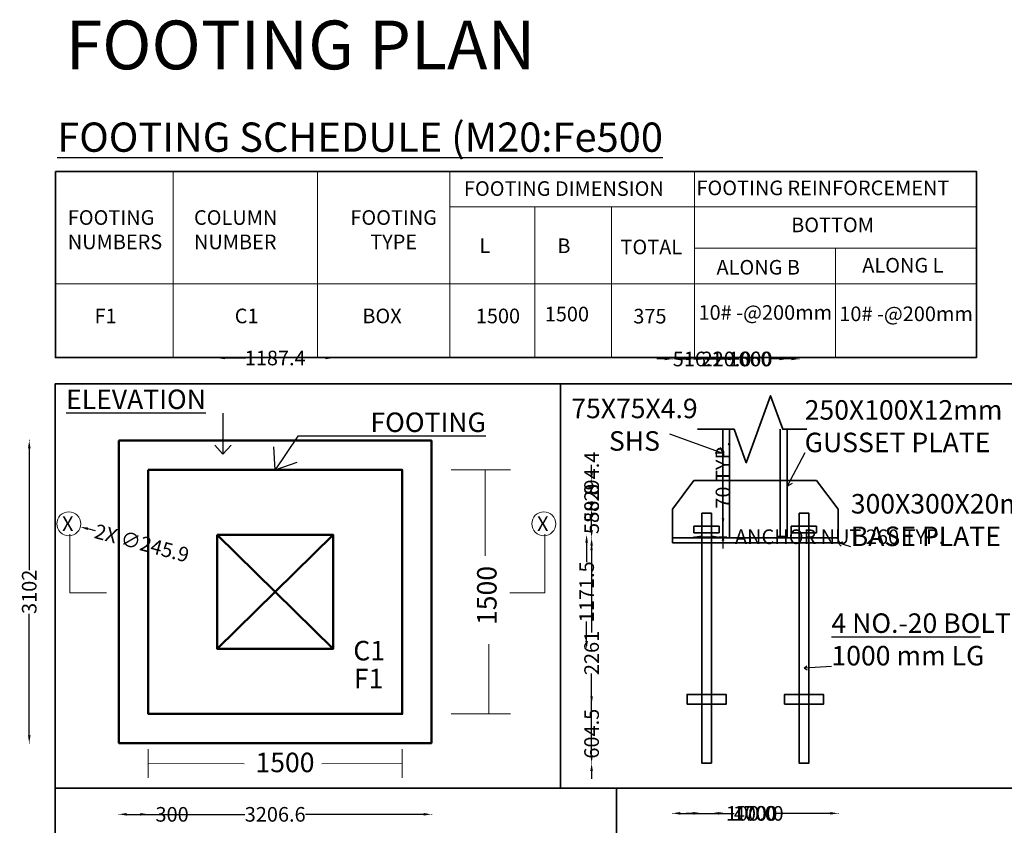
# Model space of a CAD drawing. Units: millimetres. Extents: x -19888 to 14444, y 67066 to 90098.
# Tile 2 of 7: x -19617 to -9513, y 73856 to 82117. Entities that reach past the tile are written whole.
import ezdxf

# ---------------------------------------------------------------- set-up
doc = ezdxf.new("R2010")
doc.units = ezdxf.units.MM
doc.header["$LTSCALE"] = 50
doc.header["$MEASUREMENT"] = 0
for name, color, linetype, lineweight in [('S-ANNO-DIMS', 2, 'Continuous', 18), ('S-ANNO-SYMB', 3, 'Continuous', 18), ('S-ANNO-TABL', 7, 'Continuous', 18), ('S-ANNO-TEXT', 7, 'Continuous', 25), ('S-ANNO-TTLB', 7, 'Continuous', 35), ('S-COLS', 4, 'Continuous', 50), ('S-FNDN', 1, 'Continuous', 50), ('S-STEL', 5, 'Continuous', 35)]:
    doc.layers.add(name, color=color, linetype=linetype, lineweight=lineweight)
doc.styles.get("Standard").update_dxf_attribs({"font": 'arial.ttf'})
doc.dimstyles.get("Standard").update_dxf_attribs({"dimtxt": 150, "dimasz": 80, "dimexe": 0.18, "dimexo": 0.0625, "dimgap": 0.09, "dimtad": 0, "dimdec": 0, "dimzin": 0, "dimdsep": 46, "dimtxsty": 'Standard', "dimcen": 0.09, "dimadec": 0, "dimazin": 0, "dimtfac": 1, "dimtdec": 0, "dimtofl": 0, "dimtmove": 0, "dimatfit": 3, "dimfxl": 1, "dimfxlon": 1, "dimtolj": 1, "dimtzin": 0, "dimarcsym": 0})

# ---------------------------------------------------------------- blocks, each defined once
blk = doc.blocks.new('ANCHOR-NUT')
at = {"ltscale": 50}
for p, q in [((0, 70), (0, 20)), ((80, 70), (0, 70)), ((0, 20), (0, 0)), ((0, 0), (180, 0)), ((260, 70), (80, 70)), ((180, 0), (260, 0)), ((260, 0), (260, 70))]:
    blk.add_line(p, q, dxfattribs=at)
blk = doc.blocks.new('*D22')
at = {"layer": 'Defpoints', "color": 0, "ltscale": 50, "transparency": 16777216}
for p in [(-12699, 76854), (-12439, 76854), (-12439, 76815)]:
    blk.add_point(p, dxfattribs=at)
at = {"layer": 'S-ANNO-DIMS', "color": 0, "lineweight": -2, "ltscale": 50, "transparency": 16777216}
for p, q in [((-12699, 76816), (-12699, 76815)), ((-12619, 76815), (-12519, 76815)), ((-12439, 76816), (-12439, 76815)), ((-12439, 76815), (-12359, 76815))]:
    blk.add_line(p, q, dxfattribs=at)
at = {"layer": 'S-ANNO-DIMS', "color": 0, "ltscale": 50, "transparency": 16777216}
for points in [[(-12619, 76828), (-12619, 76802), (-12699, 76815)], [(-12519, 76828), (-12519, 76802), (-12439, 76815)]]:
    blk.add_solid(points, dxfattribs=at)
at = {"layer": 'S-ANNO-DIMS', "color": 0, "ltscale": 50, "transparency": 16777216, "insert": (-11203, 76815), "char_height": 150, "attachment_point": 5}
blk.add_mtext('\\A1;ANCHOR NUT 260 TYP.', dxfattribs=at)
blk = doc.blocks.new('*D23')
at = {"layer": 'Defpoints', "color": 0, "ltscale": 50, "transparency": 16777216}
for p in [(-12439, 76924), (-12400, 76924), (-12439, 76854)]:
    blk.add_point(p, dxfattribs=at)
at = {"layer": 'S-ANNO-DIMS', "color": 0, "lineweight": -2, "ltscale": 50, "transparency": 16777216}
for p, q in [((-12400, 77004), (-12400, 77084)), ((-12401, 76924), (-12399, 76924)), ((-12401, 76854), (-12399, 76854)), ((-12400, 76774), (-12400, 76694))]:
    blk.add_line(p, q, dxfattribs=at)
at = {"layer": 'S-ANNO-DIMS', "color": 0, "ltscale": 50, "transparency": 16777216}
for points in [[(-12413, 77004), (-12386, 77004), (-12400, 76924)], [(-12413, 76774), (-12386, 76774), (-12400, 76854)]]:
    blk.add_solid(points, dxfattribs=at)
at = {"layer": 'S-ANNO-DIMS', "color": 0, "ltscale": 50, "transparency": 16777216, "insert": (-12400, 77448), "char_height": 150, "attachment_point": 5, "rotation": 90}
blk.add_mtext('\\A1;70 TYP.', dxfattribs=at)
blk = doc.blocks.new('*D33')
at = {"layer": 'Defpoints', "color": 0, "ltscale": 50, "transparency": 16777216}
for p in [(-18599, 74699), (-15392, 74699), (-15392, 73968)]:
    blk.add_point(p, dxfattribs=at)
at = {"layer": 'S-ANNO-DIMS', "color": 0, "lineweight": -2, "ltscale": 50, "transparency": 16777216}
for p, q in [((-18599, 73969), (-18599, 73968)), ((-18519, 73968), (-17307, 73968)), ((-15472, 73968), (-16684, 73968)), ((-15392, 73969), (-15392, 73968))]:
    blk.add_line(p, q, dxfattribs=at)
at = {"layer": 'S-ANNO-DIMS', "color": 0, "ltscale": 50, "transparency": 16777216}
for points in [[(-18519, 73982), (-18519, 73955), (-18599, 73968)], [(-15472, 73982), (-15472, 73955), (-15392, 73968)]]:
    blk.add_solid(points, dxfattribs=at)
at = {"layer": 'S-ANNO-DIMS', "color": 0, "ltscale": 50, "transparency": 16777216, "insert": (-16995, 73968), "char_height": 150, "attachment_point": 5}
blk.add_mtext('\\A1;3206.6', dxfattribs=at)
blk = doc.blocks.new('*D34')
at = {"layer": 'Defpoints', "color": 0, "ltscale": 50, "transparency": 16777216}
for p in [(-18599, 77801), (-19519, 74699), (-18599, 74699)]:
    blk.add_point(p, dxfattribs=at)
at = {"layer": 'S-ANNO-DIMS', "color": 0, "lineweight": -2, "ltscale": 50, "transparency": 16777216}
for p, q in [((-19518, 77801), (-19519, 77801)), ((-19519, 77721), (-19519, 76473)), ((-19519, 74779), (-19519, 76026)), ((-19518, 74699), (-19519, 74699))]:
    blk.add_line(p, q, dxfattribs=at)
at = {"layer": 'S-ANNO-DIMS', "color": 0, "ltscale": 50, "transparency": 16777216}
for points in [[(-19532, 77721), (-19505, 77721), (-19519, 77801)], [(-19532, 74779), (-19505, 74779), (-19519, 74699)]]:
    blk.add_solid(points, dxfattribs=at)
at = {"layer": 'S-ANNO-DIMS', "color": 0, "ltscale": 50, "transparency": 16777216, "insert": (-19519, 76250), "char_height": 150, "attachment_point": 5, "rotation": 90}
blk.add_mtext('\\A1;3102', dxfattribs=at)
blk = doc.blocks.new('*D35')
at = {"layer": 'Defpoints', "color": 0, "ltscale": 50, "transparency": 16777216}
for p in [(-18299, 74999), (-18599, 74699), (-18299, 73968)]:
    blk.add_point(p, dxfattribs=at)
at = {"layer": 'S-ANNO-DIMS', "color": 0, "lineweight": -2, "ltscale": 50, "transparency": 16777216}
for p, q in [((-18599, 73969), (-18599, 73968)), ((-18519, 73968), (-18379, 73968)), ((-18299, 73969), (-18299, 73968)), ((-18299, 73968), (-18219, 73968))]:
    blk.add_line(p, q, dxfattribs=at)
at = {"layer": 'S-ANNO-DIMS', "color": 0, "ltscale": 50, "transparency": 16777216}
for points in [[(-18519, 73982), (-18519, 73955), (-18599, 73968)], [(-18379, 73982), (-18379, 73955), (-18299, 73968)]]:
    blk.add_solid(points, dxfattribs=at)
at = {"layer": 'S-ANNO-DIMS', "color": 0, "ltscale": 50, "transparency": 16777216, "insert": (-18053, 73968), "char_height": 150, "attachment_point": 5}
blk.add_mtext('\\A1;300', dxfattribs=at)
blk = doc.blocks.new('*D36')
at = {"layer": 'Defpoints', "color": 0, "ltscale": 50, "transparency": 16777216}
for p in [(-16402, 78648), (-17589, 76835), (-16402, 76835)]:
    blk.add_point(p, dxfattribs=at)
at = {"layer": 'S-ANNO-DIMS', "color": 0, "lineweight": -2, "ltscale": 50, "transparency": 16777216}
for p, q in [((-17589, 78647), (-17589, 78649)), ((-17509, 78648), (-17299, 78648)), ((-16482, 78648), (-16691, 78648)), ((-16402, 78647), (-16402, 78649))]:
    blk.add_line(p, q, dxfattribs=at)
at = {"layer": 'S-ANNO-DIMS', "color": 0, "ltscale": 50, "transparency": 16777216}
for points in [[(-17509, 78662), (-17509, 78635), (-17589, 78648)], [(-16482, 78662), (-16482, 78635), (-16402, 78648)]]:
    blk.add_solid(points, dxfattribs=at)
at = {"layer": 'S-ANNO-DIMS', "color": 0, "ltscale": 50, "transparency": 16777216, "insert": (-16995, 78648), "char_height": 150, "attachment_point": 5}
blk.add_mtext('\\A1;1187.4', dxfattribs=at)
blk = doc.blocks.new('*D37')
at = {"layer": 'Defpoints', "color": 0, "ltscale": 50, "transparency": 16777216}
for p in [(-16402, 76835), (-16402, 75664), (-13799, 75664)]:
    blk.add_point(p, dxfattribs=at)
at = {"layer": 'S-ANNO-DIMS', "color": 0, "lineweight": -2, "ltscale": 50, "transparency": 16777216}
for p, q in [((-13800, 76835), (-13799, 76835)), ((-13799, 76755), (-13799, 76554)), ((-13799, 75744), (-13799, 75945)), ((-13800, 75664), (-13799, 75664))]:
    blk.add_line(p, q, dxfattribs=at)
at = {"layer": 'S-ANNO-DIMS', "color": 0, "ltscale": 50, "transparency": 16777216}
for points in [[(-13813, 76755), (-13786, 76755), (-13799, 76835)], [(-13813, 75744), (-13786, 75744), (-13799, 75664)]]:
    blk.add_solid(points, dxfattribs=at)
at = {"layer": 'S-ANNO-DIMS', "color": 0, "ltscale": 50, "transparency": 16777216, "insert": (-13799, 76250), "char_height": 150, "attachment_point": 5, "rotation": 90}
blk.add_mtext('\\A1;1171.5', dxfattribs=at)
blk = doc.blocks.new('*D38')
at = {"layer": 'Defpoints', "color": 0, "ltscale": 50, "transparency": 16777216}
for p in [(-12919, 76754), (-11219, 76754), (-11219, 73978)]:
    blk.add_point(p, dxfattribs=at)
at = {"layer": 'S-ANNO-DIMS', "color": 0, "lineweight": -2, "ltscale": 50, "transparency": 16777216}
for p, q in [((-12919, 73979), (-12919, 73978)), ((-12839, 73978), (-12285, 73978)), ((-11299, 73978), (-11852, 73978)), ((-11219, 73979), (-11219, 73978))]:
    blk.add_line(p, q, dxfattribs=at)
at = {"layer": 'S-ANNO-DIMS', "color": 0, "ltscale": 50, "transparency": 16777216}
for points in [[(-12839, 73992), (-12839, 73965), (-12919, 73978)], [(-11299, 73992), (-11299, 73965), (-11219, 73978)]]:
    blk.add_solid(points, dxfattribs=at)
at = {"layer": 'S-ANNO-DIMS', "color": 0, "ltscale": 50, "transparency": 16777216, "insert": (-12069, 73978), "char_height": 150, "attachment_point": 5}
blk.add_mtext('\\A1;1700', dxfattribs=at)
blk = doc.blocks.new('*D39')
at = {"layer": 'Defpoints', "color": 0, "ltscale": 50, "transparency": 16777216}
for p in [(-11742, 78638), (-12402, 77917), (-11742, 77917)]:
    blk.add_point(p, dxfattribs=at)
at = {"layer": 'S-ANNO-DIMS', "color": 0, "lineweight": -2, "ltscale": 50, "transparency": 16777216}
for p, q in [((-12402, 78637), (-12402, 78639)), ((-12322, 78638), (-12238, 78638)), ((-11822, 78638), (-11906, 78638)), ((-11742, 78637), (-11742, 78639))]:
    blk.add_line(p, q, dxfattribs=at)
at = {"layer": 'S-ANNO-DIMS', "color": 0, "ltscale": 50, "transparency": 16777216}
for points in [[(-12322, 78652), (-12322, 78625), (-12402, 78638)], [(-11822, 78652), (-11822, 78625), (-11742, 78638)]]:
    blk.add_solid(points, dxfattribs=at)
at = {"layer": 'S-ANNO-DIMS', "color": 0, "ltscale": 50, "transparency": 16777216, "insert": (-12072, 78638), "char_height": 150, "attachment_point": 5}
blk.add_mtext('\\A1;660', dxfattribs=at)
blk = doc.blocks.new('*D40')
at = {"layer": 'Defpoints', "color": 0, "ltscale": 50, "transparency": 16777216}
for p in [(-11619, 78638), (-12619, 77056), (-11619, 77056)]:
    blk.add_point(p, dxfattribs=at)
at = {"layer": 'S-ANNO-DIMS', "color": 0, "lineweight": -2, "ltscale": 50, "transparency": 16777216}
for p, q in [((-12619, 78637), (-12619, 78639)), ((-12539, 78638), (-12335, 78638)), ((-11699, 78638), (-11902, 78638)), ((-11619, 78637), (-11619, 78639))]:
    blk.add_line(p, q, dxfattribs=at)
at = {"layer": 'S-ANNO-DIMS', "color": 0, "ltscale": 50, "transparency": 16777216}
for points in [[(-12539, 78652), (-12539, 78625), (-12619, 78638)], [(-11699, 78652), (-11699, 78625), (-11619, 78638)]]:
    blk.add_solid(points, dxfattribs=at)
at = {"layer": 'S-ANNO-DIMS', "color": 0, "ltscale": 50, "transparency": 16777216, "insert": (-12119, 78638), "char_height": 150, "attachment_point": 5}
blk.add_mtext('\\A1;1000', dxfattribs=at)
blk = doc.blocks.new('*D41')
at = {"layer": 'Defpoints', "color": 0, "ltscale": 50, "transparency": 16777216}
for p in [(-11742, 77917), (-8716, 77917), (-11519, 74493)]:
    blk.add_point(p, dxfattribs=at)
at = {"layer": 'S-ANNO-DIMS', "color": 0, "lineweight": -2, "ltscale": 50, "transparency": 16777216}
for p, q in [((-8717, 77917), (-8716, 77917)), ((-8716, 77837), (-8716, 76429)), ((-8716, 74573), (-8716, 75981)), ((-8717, 74493), (-8716, 74493))]:
    blk.add_line(p, q, dxfattribs=at)
at = {"layer": 'S-ANNO-DIMS', "color": 0, "ltscale": 50, "transparency": 16777216}
for points in [[(-8729, 77837), (-8703, 77837), (-8716, 77917)], [(-8729, 74573), (-8703, 74573), (-8716, 74493)]]:
    blk.add_solid(points, dxfattribs=at)
at = {"layer": 'S-ANNO-DIMS', "color": 0, "ltscale": 50, "transparency": 16777216, "insert": (-8716, 76205), "char_height": 150, "attachment_point": 5, "rotation": 90}
blk.add_mtext('\\A1;3424', dxfattribs=at)
blk = doc.blocks.new('*D42')
at = {"layer": 'Defpoints', "color": 0, "ltscale": 50, "transparency": 16777216}
for p in [(-11742, 77917), (-11219, 76804), (-8716, 76804)]:
    blk.add_point(p, dxfattribs=at)
at = {"layer": 'S-ANNO-DIMS', "color": 0, "lineweight": -2, "ltscale": 50, "transparency": 16777216}
for p, q in [((-8717, 77917), (-8716, 77917)), ((-8716, 77837), (-8716, 77665)), ((-8716, 76884), (-8716, 77056)), ((-8717, 76804), (-8716, 76804))]:
    blk.add_line(p, q, dxfattribs=at)
at = {"layer": 'S-ANNO-DIMS', "color": 0, "ltscale": 50, "transparency": 16777216}
for points in [[(-8729, 77837), (-8703, 77837), (-8716, 77917)], [(-8729, 76884), (-8703, 76884), (-8716, 76804)]]:
    blk.add_solid(points, dxfattribs=at)
at = {"layer": 'S-ANNO-DIMS', "color": 0, "ltscale": 50, "transparency": 16777216, "insert": (-8716, 77360), "char_height": 150, "attachment_point": 5, "rotation": 90}
blk.add_mtext('\\A1;1112.9', dxfattribs=at)
blk = doc.blocks.new('*D43')
at = {"layer": 'Defpoints', "color": 0, "ltscale": 50, "transparency": 16777216}
for p in [(-13748, 77393), (-12699, 77393), (-12919, 76804)]:
    blk.add_point(p, dxfattribs=at)
at = {"layer": 'S-ANNO-DIMS', "color": 0, "lineweight": -2, "ltscale": 50, "transparency": 16777216}
for p, q in [((-13748, 77473), (-13748, 77553)), ((-13747, 77393), (-13748, 77393)), ((-13747, 76804), (-13748, 76804)), ((-13748, 76724), (-13748, 76644))]:
    blk.add_line(p, q, dxfattribs=at)
at = {"layer": 'S-ANNO-DIMS', "color": 0, "ltscale": 50, "transparency": 16777216}
for points in [[(-13761, 77473), (-13735, 77473), (-13748, 77393)], [(-13761, 76724), (-13735, 76724), (-13748, 76804)]]:
    blk.add_solid(points, dxfattribs=at)
at = {"layer": 'S-ANNO-DIMS', "color": 0, "ltscale": 50, "transparency": 16777216, "insert": (-13748, 77098), "char_height": 150, "attachment_point": 5, "rotation": 90}
blk.add_mtext('\\A1;588.8', dxfattribs=at)
blk = doc.blocks.new('*D44')
at = {"layer": 'Defpoints', "color": 0, "ltscale": 50, "transparency": 16777216}
for p in [(-13748, 76754), (-12919, 76754), (-12619, 74493)]:
    blk.add_point(p, dxfattribs=at)
at = {"layer": 'S-ANNO-DIMS', "color": 0, "lineweight": -2, "ltscale": 50, "transparency": 16777216}
for p, q in [((-13747, 76754), (-13748, 76754)), ((-13748, 76674), (-13748, 75834)), ((-13748, 74573), (-13748, 75413)), ((-13747, 74493), (-13748, 74493))]:
    blk.add_line(p, q, dxfattribs=at)
at = {"layer": 'S-ANNO-DIMS', "color": 0, "ltscale": 50, "transparency": 16777216}
for points in [[(-13761, 76674), (-13735, 76674), (-13748, 76754)], [(-13761, 74573), (-13735, 74573), (-13748, 74493)]]:
    blk.add_solid(points, dxfattribs=at)
at = {"layer": 'S-ANNO-DIMS', "color": 0, "ltscale": 50, "transparency": 16777216, "insert": (-13748, 75623), "char_height": 150, "attachment_point": 5, "rotation": 90}
blk.add_mtext('\\A1;2261', dxfattribs=at)
blk = doc.blocks.new('*D45')
at = {"layer": 'Defpoints', "color": 0, "ltscale": 50, "transparency": 16777216}
for p in [(-12769, 75098), (-13748, 74493), (-12619, 74493)]:
    blk.add_point(p, dxfattribs=at)
at = {"layer": 'S-ANNO-DIMS', "color": 0, "lineweight": -2, "ltscale": 50, "transparency": 16777216}
for p, q in [((-13748, 75178), (-13748, 75258)), ((-13747, 75098), (-13748, 75098)), ((-13747, 74493), (-13748, 74493)), ((-13748, 74413), (-13748, 74333))]:
    blk.add_line(p, q, dxfattribs=at)
at = {"layer": 'S-ANNO-DIMS', "color": 0, "ltscale": 50, "transparency": 16777216}
for points in [[(-13761, 75178), (-13735, 75178), (-13748, 75098)], [(-13761, 74413), (-13735, 74413), (-13748, 74493)]]:
    blk.add_solid(points, dxfattribs=at)
at = {"layer": 'S-ANNO-DIMS', "color": 0, "ltscale": 50, "transparency": 16777216, "insert": (-13748, 74795), "char_height": 150, "attachment_point": 5, "rotation": 90}
blk.add_mtext('\\A1;604.5', dxfattribs=at)
blk = doc.blocks.new('*D90')
at = {"layer": 'Defpoints', "color": 0, "ltscale": 50, "transparency": 16777216}
for p in [(-13748, 77098), (-12919, 77098), (-12919, 76804)]:
    blk.add_point(p, dxfattribs=at)
at = {"layer": 'S-ANNO-DIMS', "color": 0, "lineweight": -2, "ltscale": 50, "transparency": 16777216}
for p, q in [((-13748, 77098), (-13748, 77178)), ((-13747, 77098), (-13748, 77098)), ((-13748, 76884), (-13748, 77018)), ((-13747, 76804), (-13748, 76804))]:
    blk.add_line(p, q, dxfattribs=at)
at = {"layer": 'S-ANNO-DIMS', "color": 0, "ltscale": 50, "transparency": 16777216}
for points in [[(-13761, 77018), (-13735, 77018), (-13748, 77098)], [(-13761, 76884), (-13735, 76884), (-13748, 76804)]]:
    blk.add_solid(points, dxfattribs=at)
at = {"layer": 'S-ANNO-DIMS', "color": 0, "ltscale": 50, "transparency": 16777216, "insert": (-13748, 77432), "char_height": 150, "attachment_point": 5, "rotation": 90}
blk.add_mtext('\\A1;294.4', dxfattribs=at)
blk = doc.blocks.new('*D91')
at = {"layer": 'Defpoints', "color": 0, "ltscale": 50, "transparency": 16777216}
for p in [(-12699, 78638), (-12699, 77393), (-12919, 77098)]:
    blk.add_point(p, dxfattribs=at)
at = {"layer": 'S-ANNO-DIMS', "color": 0, "lineweight": -2, "ltscale": 50, "transparency": 16777216}
for p, q in [((-12919, 78637), (-12919, 78639)), ((-12839, 78638), (-12779, 78638)), ((-12699, 78637), (-12699, 78639)), ((-12699, 78638), (-12619, 78638))]:
    blk.add_line(p, q, dxfattribs=at)
at = {"layer": 'S-ANNO-DIMS', "color": 0, "ltscale": 50, "transparency": 16777216}
for points in [[(-12839, 78652), (-12839, 78625), (-12919, 78638)], [(-12779, 78652), (-12779, 78625), (-12699, 78638)]]:
    blk.add_solid(points, dxfattribs=at)
at = {"layer": 'S-ANNO-DIMS', "color": 0, "ltscale": 50, "transparency": 16777216, "insert": (-12364, 78638), "char_height": 150, "attachment_point": 5}
blk.add_mtext('\\A1;220.0', dxfattribs=at)
blk = doc.blocks.new('*D92')
at = {"layer": 'Defpoints', "color": 0, "ltscale": 50, "transparency": 16777216}
for p in [(-12402, 78638), (-12402, 77917), (-12919, 76804)]:
    blk.add_point(p, dxfattribs=at)
at = {"layer": 'S-ANNO-DIMS', "color": 0, "lineweight": -2, "ltscale": 50, "transparency": 16777216}
for p, q in [((-12999, 78638), (-13079, 78638)), ((-12919, 78637), (-12919, 78639)), ((-12402, 78637), (-12402, 78639)), ((-12322, 78638), (-12242, 78638))]:
    blk.add_line(p, q, dxfattribs=at)
at = {"layer": 'S-ANNO-DIMS', "color": 0, "ltscale": 50, "transparency": 16777216}
for points in [[(-12999, 78652), (-12999, 78625), (-12919, 78638)], [(-12322, 78652), (-12322, 78625), (-12402, 78638)]]:
    blk.add_solid(points, dxfattribs=at)
at = {"layer": 'S-ANNO-DIMS', "color": 0, "ltscale": 50, "transparency": 16777216, "insert": (-12660, 78638), "char_height": 150, "attachment_point": 5}
blk.add_mtext('\\A1;516.1', dxfattribs=at)
blk = doc.blocks.new('*D93')
at = {"layer": 'Defpoints', "color": 0, "ltscale": 50, "transparency": 16777216}
for p in [(-12769, 75098), (-12369, 75098), (-12369, 73978)]:
    blk.add_point(p, dxfattribs=at)
at = {"layer": 'S-ANNO-DIMS', "color": 0, "lineweight": -2, "ltscale": 50, "transparency": 16777216}
for p, q in [((-12769, 73979), (-12769, 73978)), ((-12689, 73978), (-12449, 73978)), ((-12369, 73979), (-12369, 73978)), ((-12369, 73978), (-12289, 73978))]:
    blk.add_line(p, q, dxfattribs=at)
at = {"layer": 'S-ANNO-DIMS', "color": 0, "ltscale": 50, "transparency": 16777216}
for points in [[(-12689, 73992), (-12689, 73965), (-12769, 73978)], [(-12449, 73992), (-12449, 73965), (-12369, 73978)]]:
    blk.add_solid(points, dxfattribs=at)
at = {"layer": 'S-ANNO-DIMS', "color": 0, "ltscale": 50, "transparency": 16777216, "insert": (-12033, 73978), "char_height": 150, "attachment_point": 5}
blk.add_mtext('\\A1;400.0', dxfattribs=at)
blk = doc.blocks.new('*D94')
at = {"layer": 'Defpoints', "color": 0, "ltscale": 50, "transparency": 16777216}
for p in [(-11369, 75198), (-8716, 75198), (-11369, 75098)]:
    blk.add_point(p, dxfattribs=at)
at = {"layer": 'S-ANNO-DIMS', "color": 0, "lineweight": -2, "ltscale": 50, "transparency": 16777216}
for p, q in [((-8716, 75278), (-8716, 75358)), ((-8717, 75198), (-8716, 75198)), ((-8717, 75098), (-8716, 75098)), ((-8716, 75018), (-8716, 74938))]:
    blk.add_line(p, q, dxfattribs=at)
at = {"layer": 'S-ANNO-DIMS', "color": 0, "ltscale": 50, "transparency": 16777216}
for points in [[(-8729, 75278), (-8703, 75278), (-8716, 75198)], [(-8729, 75018), (-8703, 75018), (-8716, 75098)]]:
    blk.add_solid(points, dxfattribs=at)
at = {"layer": 'S-ANNO-DIMS', "color": 0, "ltscale": 50, "transparency": 16777216, "insert": (-8716, 75603), "char_height": 150, "attachment_point": 5, "rotation": 90}
blk.add_mtext('\\A1;100.0', dxfattribs=at)
blk = doc.blocks.new('*D95')
at = {"layer": 'Defpoints', "color": 0, "ltscale": 50, "transparency": 16777216}
for p in [(-12619, 74493), (-12519, 74493), (-12519, 73978)]:
    blk.add_point(p, dxfattribs=at)
at = {"layer": 'S-ANNO-DIMS', "color": 0, "lineweight": -2, "ltscale": 50, "transparency": 16777216}
for p, q in [((-12699, 73978), (-12779, 73978)), ((-12619, 73979), (-12619, 73978)), ((-12519, 73979), (-12519, 73978)), ((-12439, 73978), (-12359, 73978))]:
    blk.add_line(p, q, dxfattribs=at)
at = {"layer": 'S-ANNO-DIMS', "color": 0, "ltscale": 50, "transparency": 16777216}
for points in [[(-12699, 73992), (-12699, 73965), (-12619, 73978)], [(-12439, 73992), (-12439, 73965), (-12519, 73978)]]:
    blk.add_solid(points, dxfattribs=at)
at = {"layer": 'S-ANNO-DIMS', "color": 0, "ltscale": 50, "transparency": 16777216, "insert": (-12113, 73978), "char_height": 150, "attachment_point": 5}
blk.add_mtext('\\A1;100.0', dxfattribs=at)
blk = doc.blocks.new('*D96')
at = {"layer": 'Defpoints', "color": 0, "ltscale": 50, "transparency": 16777216}
for p in [(-13748, 76804), (-12919, 76804), (-12919, 76754)]:
    blk.add_point(p, dxfattribs=at)
at = {"layer": 'S-ANNO-DIMS', "color": 0, "lineweight": -2, "ltscale": 50, "transparency": 16777216}
for p, q in [((-13748, 76884), (-13748, 76964)), ((-13747, 76804), (-13748, 76804)), ((-13747, 76754), (-13748, 76754)), ((-13748, 76674), (-13748, 76594))]:
    blk.add_line(p, q, dxfattribs=at)
at = {"layer": 'S-ANNO-DIMS', "color": 0, "ltscale": 50, "transparency": 16777216}
for points in [[(-13761, 76884), (-13735, 76884), (-13748, 76804)], [(-13761, 76674), (-13735, 76674), (-13748, 76754)]]:
    blk.add_solid(points, dxfattribs=at)
at = {"layer": 'S-ANNO-DIMS', "color": 0, "ltscale": 50, "transparency": 16777216, "insert": (-13748, 77159), "char_height": 150, "attachment_point": 5, "rotation": 90}
blk.add_mtext('\\A1;50.0', dxfattribs=at)
blk = doc.blocks.new('*D102')
at = {"layer": 'Defpoints', "color": 0, "ltscale": 50, "transparency": 16777216}
for p in [(-19232, 76980), (-18995, 76917)]:
    blk.add_point(p, dxfattribs=at)
at = {"layer": 'S-ANNO-DIMS', "color": 0, "lineweight": -2, "ltscale": 50, "transparency": 16777216}
for p, q in [((-19113, 76948), (-19113, 76948)), ((-19113, 76948), (-19113, 76948)), ((-18840, 76875), (-18917, 76896))]:
    blk.add_line(p, q, dxfattribs=at)
at = {"layer": 'S-ANNO-DIMS', "color": 0, "ltscale": 50, "transparency": 16777216}
blk.add_solid([(-18914, 76909), (-18921, 76883), (-18995, 76917)], dxfattribs=at)
at = {"layer": 'S-ANNO-DIMS', "color": 0, "ltscale": 50, "transparency": 16777216, "insert": (-18363, 76749), "char_height": 150, "attachment_point": 5, "rotation": 345.1105}
blk.add_mtext('\\A1;2X ∅245.9', dxfattribs=at)

msp = doc.modelspace()

# ---------------------------------------------------------------- linework, layer by layer
at = {"layer": 'S-ANNO-DIMS', "ltscale": 50}
for p, q in [((-15190.147, 77500.576), (-14580.674, 77500.576)), ((-14840.514, 76619.359), (-14840.514, 77500.576)), ((-14803.107, 75713.38), (-14803.107, 74998.52)), ((-15190.147, 74998.52), (-14580.674, 74998.52)), ((-18298.527, 74635.878), (-18298.527, 74341.123)), ((-15691.95, 74635.878), (-15691.95, 74341.123)), ((-17314.587, 74487.219), (-18298.527, 74488.5)), ((-16517.745, 74487.219), (-15691.95, 74488.5))]:
    msp.add_line(p, q, dxfattribs=at)
at = {"layer": 'S-ANNO-SYMB', "ltscale": 50}
for p, q in [((-19102.21, 76239.701), (-19102.21, 76841.262)), ((-14227.686, 76239.701), (-14227.686, 76841.262)), ((-18724.539, 76239.701), (-19102.21, 76239.701)), ((-14585.822, 76239.701), (-14227.686, 76239.701))]:
    msp.add_line(p, q, dxfattribs=at)
for centre in [(-19113.353, 76948.115), (-14238.829, 76948.115)]:
    msp.add_circle(centre, 122.945, dxfattribs=at)
at = {"layer": 'S-ANNO-TABL', "ltscale": 50}
for p, q in [((-18040.466, 80561.742), (-18040.466, 78652.531)), ((-16560.262, 80561.742), (-16560.262, 78652.531)), ((-15203.409, 80561.742), (-15203.409, 78652.531)), ((-12691.473, 80561.742), (-12691.473, 78652.531)), ((-15203.409, 80198.629), (-9798.872, 80198.629)), ((-14332.194, 80198.629), (-14332.194, 78652.531)), ((-13543.386, 80198.629), (-13543.386, 78652.531)), ((-12691.473, 79772.886), (-9798.872, 79772.886)), ((-11245.173, 79772.886), (-11245.173, 78652.531)), ((-19249.942, 79409.181), (-15203.409, 79409.181)), ((-15203.409, 79409.181), (-9798.872, 79409.181))]:
    msp.add_line(p, q, dxfattribs=at)
at = {"layer": 'S-ANNO-TEXT', "ltscale": 50}
for p, q in [((-17531.763, 78081.147), (-17531.763, 77662.054)), ((-16763.898, 77845.451), (-16995.238, 77500.576)), ((-16017.716, 77845.451), (-16763.898, 77845.451)), ((-12947.831, 77868.665), (-12402.365, 77671.319)), ((-17531.763, 77662.054), (-17615.599, 77753.443)), ((-17531.763, 77662.054), (-17447.927, 77753.443)), ((-16995.238, 77500.576), (-17008.58, 77737.797)), ((-12402.365, 77671.319), (-12426.678, 77729.901)), ((-12402.365, 77671.319), (-12478.636, 77671.863)), ((-11561.522, 77674.531), (-11742.33, 77333.859)), ((-16995.238, 77500.576), (-16770.687, 77578.219)), ((-11742.33, 77333.859), (-11737.562, 77391.137)), ((-11742.33, 77333.859), (-11686.135, 77364.305)), ((-11218.513, 76753.857), (-11171.568, 76763.997)), ((-11088.137, 76711.8), (-11218.513, 76753.857)), ((-11218.513, 76753.857), (-11186.342, 76718.196)), ((-11565.74, 75468.599), (-11538.539, 75490.227)), ((-11286.71, 75485.058), (-11565.74, 75468.599)), ((-11565.74, 75468.599), (-11536.186, 75450.319))]:
    msp.add_line(p, q, dxfattribs=at)
at = {"layer": 'S-ANNO-TTLB', "ltscale": 50}
for points in [[(-19249.942, 80561.742), (-9798.872, 80561.742), (-9798.872, 78652.531), (-19249.942, 78652.531)], [(-19251.506, 78381.341), (-14066.3, 78381.341), (-14066.3, 74235.431), (-19251.506, 74235.431)], [(-14066.3, 78381.341), (-8972.922, 78381.341), (-8972.922, 74235.431), (-14066.3, 74235.431)], [(-19251.506, 74235.431), (-13491.006, 74235.431), (-13491.006, 69226.696), (-19251.506, 69226.696)], [(-13491.006, 74235.431), (-9009.653, 74235.431), (-9009.653, 69226.696), (-13491.006, 69226.696)]]:
    msp.add_lwpolyline(points, close=True, dxfattribs=at)
at = {"layer": 'S-COLS', "ltscale": 50}
for p, q in [((-17588.959, 76835.289), (-16401.518, 75663.806)), ((-17588.959, 75663.806), (-16401.518, 76835.289))]:
    msp.add_line(p, q, dxfattribs=at)
msp.add_lwpolyline([(-17588.959, 76835.289), (-16401.518, 76835.289), (-16401.518, 75663.806), (-17588.959, 75663.806)], close=True, dxfattribs=at)
at = {"layer": 'S-FNDN', "ltscale": 50}
for points in [[(-18598.527, 77800.576), (-15391.95, 77800.576), (-15391.95, 74698.52), (-18598.527, 74698.52)], [(-18298.527, 77500.576), (-15691.95, 77500.576), (-15691.95, 74998.52), (-18298.527, 74998.52)]]:
    msp.add_lwpolyline(points, close=True, dxfattribs=at)
at = {"layer": 'S-STEL', "ltscale": 50}
for p, q in [((-12402.365, 76803.857), (-12402.365, 77916.725)), ((-12332.365, 76803.857), (-12332.365, 77916.725)), ((-11812.33, 76803.857), (-11812.33, 77916.725)), ((-11742.33, 76803.857), (-11742.33, 77916.725)), ((-12918.513, 77098.246), (-12698.513, 77392.635)), ((-12698.513, 77392.635), (-11438.513, 77392.635)), ((-11218.513, 77098.246), (-11438.513, 77392.635)), ((-12918.513, 76803.857), (-12918.513, 77098.246)), ((-11218.513, 76803.857), (-11218.513, 77098.246)), ((-12918.513, 76803.857), (-12698.513, 76803.857)), ((-12918.513, 76803.857), (-12918.513, 76753.857)), ((-12438.513, 76803.857), (-12698.513, 76803.857)), ((-12438.513, 76803.857), (-11698.513, 76803.857)), ((-11518.513, 76803.857), (-11698.513, 76803.857)), ((-11518.513, 76803.857), (-11218.513, 76803.857)), ((-11218.513, 76803.857), (-11218.513, 76753.857)), ((-11218.513, 76753.857), (-12918.513, 76753.857))]:
    msp.add_line(p, q, dxfattribs=at)
msp.add_lwpolyline([(-12662.035, 77916.725), (-12286.395, 77916.725), (-12161.395, 77573.29), (-11911.395, 78260.16), (-11786.395, 77916.725), (-11540.385, 77916.725)], dxfattribs=at)
for points in [[(-12618.513, 77055.765), (-12518.513, 77055.765), (-12518.513, 74493.06), (-12618.513, 74493.06)], [(-11618.513, 77055.765), (-11518.513, 77055.765), (-11518.513, 74493.06), (-11618.513, 74493.06)], [(-12768.513, 75097.57), (-12768.513, 75197.57), (-12518.513, 75197.57), (-12368.513, 75197.57), (-12368.513, 75097.57), (-12618.513, 75097.57)], [(-11768.513, 75097.57), (-11768.513, 75197.57), (-11518.513, 75197.57), (-11368.513, 75197.57), (-11368.513, 75097.57), (-11618.513, 75097.57)]]:
    msp.add_lwpolyline(points, close=True, dxfattribs=at)

# ---------------------------------------------------------------- block references
at = {"layer": 'S-STEL'}
for p in [(-12698.513, 76853.857), (-11698.513, 76853.857)]:
    msp.add_blockref('ANCHOR-NUT', p, dxfattribs=at)

# ---------------------------------------------------------------- texts
at = {"layer": 'S-ANNO-TEXT', "ltscale": 50, "attachment_point": 1}
for s, width, insert, char_height in [('FOOTING PLAN', 5845.79275, (-19146.941, 82108.435), 500), ('{\\LFOOTING SCHEDULE (M20:Fe500}', 11373.05188, (-19232.163, 81062.74), 300), ('FOOTING DIMENSION', 2684.68082, (-15057.932, 80460.534), 150), ('FOOTING REINFORCEMENT', 3143.26265, (-12671.901, 80467.425), 150), ('FOOTING \\PNUMBERS', 11373.05188, (-19123.342, 80163.582), 150), ('COLUMN NUMBER', 1590.49887, (-17828.289, 80163.582), 150), ('\\pxqc;FOOTING\\PTYPE', 11373.05188, (-21465.754, 80163.582), 150), ('BOTTOM', 11373.05188, (-11700.149, 80087.995), 150), ('L ', 1590.49887, (-14900.122, 79876.338), 150), ('B', 1590.49887, (-14099.475, 79874.067), 150), ('TOTAL', 1590.49887, (-13451.679, 79861.704), 150), ('ALONG B', 11373.05188, (-12466.28, 79653.418), 150), ('ALONG L', 11373.05188, (-10970.497, 79674.333), 150), ('F1', 11373.05188, (-18848.715, 79154.148), 150), ('C1', 11373.05188, (-17410.511, 79154.148), 150), ('BOX', 11373.05188, (-16100.718, 79154.148), 150), ('1500', 11373.05188, (-14936.458, 79154.148), 150), ('1500', 11373.05188, (-14228.81, 79173.8), 150), ('375', 11373.05188, (-13319.885, 79152.004), 150), ('10# -@200mm', 11373.05188, (-12650.912, 79189.732), 150), ('10# -@200mm', 11373.05188, (-11206.153, 79175.946), 150), ('{\\LELEVATION}', 1609.35955, (-19141.123, 78324.695), 200), ('\\pxqc;75X75X4.9\\PSHS', 1609.35955, (-14112.977, 78230.496), 200), ('250X100X12mm\\PGUSSET PLATE', 2123.78165, (-11561.522, 78215.504), 200), ('{\\LFOOTING}', 1609.35955, (-16017.716, 78088.998), 200), ('300X300X20mm\\PBASE PLATE', 2233.4119, (-11088.137, 77252.773), 200), ('X', 11373.05188, (-19182.112, 77023.115), 150), ('X', 11373.05188, (-14307.588, 77023.115), 150), ('{\\L4 NO.-20 BO}LTS\\P1000 mm LG', 2263.41642, (-11286.71, 76028.76), 200), ('C1', 1609.35955, (-16193.471, 75747.035), 200), ('F1', 1609.35955, (-16187.768, 75460.345), 200), ('1500', 1609.35955, (-17197.407, 74600.266), 200)]:
    msp.add_mtext_dynamic_manual_height_columns(s, width=width, gutter_width=1, heights=[0], dxfattribs=dict(at, insert=insert, char_height=char_height))
at = {"layer": 'S-ANNO-TEXT', "ltscale": 50, "insert": (-14923.171, 75909.52), "char_height": 200, "attachment_point": 1, "rotation": 90}
msp.add_mtext_dynamic_manual_height_columns('1500', width=1609.35955, gutter_width=1, heights=[0], dxfattribs=at)

# ---------------------------------------------------------------- dimensions: what is measured, and where the dimension line sits
at = {"layer": 'S-ANNO-DIMS', "ltscale": 50}
for base, p1, p2, override, picture, middle in [((-16401.518, 78648.341), (-17588.959, 76835.289), (-16401.518, 76835.289), {"dimdec": 1, "dimlfac": 1, "dimrnd": 0, "dimzin": 0, "dimdsep": 46, "dimlunit": 2}, '*D36', (-16995.238, 78648.341)), ((-12402.365, 78638.341), (-12918.513, 76803.857), (-12402.365, 77916.725), {"dimdec": 1, "dimlfac": 1, "dimrnd": 0, "dimzin": 0, "dimdsep": 46, "dimlunit": 2}, '*D92', (-12660.439, 78638.341)), ((-12698.513, 78638.341), (-12918.513, 77098.246), (-12698.513, 77392.635), {"dimdec": 1, "dimlfac": 1, "dimrnd": 0, "dimzin": 0, "dimdsep": 46, "dimlunit": 2}, '*D91', (-12364.313, 78638.341)), ((-11618.513, 78638.341), (-12618.513, 77055.765), (-11618.513, 77055.765), {"dimdec": 0, "dimlfac": 1, "dimrnd": 0, "dimzin": 0, "dimdsep": 46, "dimlunit": 2}, '*D40', (-12118.513, 78638.341)), ((-11742.33, 78638.341), (-12402.365, 77916.725), (-11742.33, 77916.725), {"dimdec": 0, "dimlfac": 1, "dimrnd": 0, "dimzin": 0, "dimdsep": 46, "dimlunit": 2}, '*D39', (-12072.348, 78638.341)), ((-11218.513, 73978.431), (-12918.513, 76753.857), (-11218.513, 76753.857), {"dimdec": 0, "dimlfac": 1, "dimrnd": 0, "dimzin": 0, "dimdsep": 46, "dimlunit": 2}, '*D38', (-12068.513, 73978.431)), ((-12368.513, 73978.431), (-12768.513, 75097.57), (-12368.513, 75097.57), {"dimdec": 1, "dimlfac": 1, "dimrnd": 0, "dimzin": 0, "dimdsep": 46, "dimlunit": 2}, '*D93', (-12032.574, 73978.431)), ((-18298.527, 73968.431), (-18598.527, 74698.52), (-18298.527, 74998.52), {"dimdec": 0, "dimlfac": 1, "dimrnd": 0, "dimzin": 0, "dimdsep": 46, "dimlunit": 2}, '*D35', (-18053.038, 73968.431)), ((-15391.95, 73968.431), (-18598.527, 74698.52), (-15391.95, 74698.52), {"dimdec": 1, "dimlfac": 1, "dimrnd": 0, "dimzin": 0, "dimdsep": 46, "dimlunit": 2}, '*D33', (-16995.238, 73968.431)), ((-12518.513, 73978.431), (-12618.513, 74493.06), (-12518.513, 74493.06), {"dimdec": 1, "dimlfac": 1, "dimrnd": 0, "dimzin": 0, "dimdsep": 46, "dimlunit": 2}, '*D95', (-12112.652, 73978.431))]:
    dim = msp.add_linear_dim(base=base, p1=p1, p2=p2, dimstyle='Standard', override=override, dxfattribs=at)
    dim.commit()
    dim.dimension.update_dxf_attribs({"geometry": picture, "text_midpoint": middle})
for base, p1, p2, override, picture, middle in [((-8715.922, 77916.725), (-11518.513, 74493.06), (-11742.33, 77916.725), {"dimdec": 0, "dimlfac": 1, "dimrnd": 0, "dimzin": 0, "dimdsep": 46, "dimlunit": 2}, '*D41', (-8715.922, 76204.893)), ((-8715.922, 76803.857), (-11742.33, 77916.725), (-11218.513, 76803.857), {"dimdec": 1, "dimlfac": 1, "dimrnd": 0, "dimzin": 0, "dimdsep": 46, "dimlunit": 2}, '*D42', (-8715.922, 77360.291)), ((-19518.506, 74698.52), (-18598.527, 77800.576), (-18598.527, 74698.52), {"dimdec": 0, "dimlfac": 1, "dimrnd": 0, "dimzin": 0, "dimdsep": 46, "dimlunit": 2}, '*D34', (-19518.506, 76249.548)), ((-13748.006, 77098.246), (-12918.513, 76803.857), (-12918.513, 77098.246), {"dimdec": 1, "dimlfac": 1, "dimrnd": 0, "dimzin": 0, "dimdsep": 46, "dimlunit": 2}, '*D90', (-13748.006, 77432.395)), ((-13748.006, 77392.635), (-12918.513, 76803.857), (-12698.513, 77392.635), {"dimdec": 1, "dimlfac": 1, "dimrnd": 0, "dimzin": 0, "dimdsep": 46, "dimlunit": 2}, '*D43', (-13748.006, 77098.246)), ((-13748.006, 76803.857), (-12918.513, 76753.857), (-12918.513, 76803.857), {"dimdec": 1, "dimlfac": 1, "dimrnd": 0, "dimzin": 0, "dimdsep": 46, "dimlunit": 2}, '*D96', (-13748.006, 77158.508)), ((-13799.3, 75663.806), (-16401.518, 76835.289), (-16401.518, 75663.806), {"dimdec": 1, "dimlfac": 1, "dimrnd": 0, "dimzin": 0, "dimdsep": 46, "dimlunit": 2}, '*D37', (-13799.3, 76249.548)), ((-13748.006, 76753.857), (-12618.513, 74493.06), (-12918.513, 76753.857), {"dimdec": 0, "dimlfac": 1, "dimrnd": 0, "dimzin": 0, "dimdsep": 46, "dimlunit": 2}, '*D44', (-13748.006, 75623.459)), ((-8715.922, 75197.57), (-11368.513, 75097.57), (-11368.513, 75197.57), {"dimdec": 1, "dimlfac": 1, "dimrnd": 0, "dimzin": 0, "dimdsep": 46, "dimlunit": 2}, '*D94', (-8715.922, 75603.431)), ((-13748.006, 74493.06), (-12768.513, 75097.57), (-12618.513, 74493.06), {"dimdec": 1, "dimlfac": 1, "dimrnd": 0, "dimzin": 0, "dimdsep": 46, "dimlunit": 2}, '*D45', (-13748.006, 74795.315))]:
    dim = msp.add_linear_dim(base=base, p1=p1, p2=p2, angle=90, dimstyle='Standard', override=override, dxfattribs=at)
    dim.commit()
    dim.dimension.update_dxf_attribs({"geometry": picture, "text_midpoint": middle})
dim = msp.add_linear_dim(base=(-12399.513, 76923.857), p1=(-12438.513, 76853.857), p2=(-12438.513, 76923.857), angle=90, text='<> TYP.', dimstyle='Standard', override={"dimdec": 0, "dimrnd": 0, "dimzin": 0, "dimlunit": 2}, dxfattribs=at)
dim.commit()
dim.dimension.update_dxf_attribs({"geometry": '*D23', "text_midpoint": (-12399.513, 77448.409)})
dim = msp.add_linear_dim(base=(-12438.513, 76814.857), p1=(-12698.513, 76853.857), p2=(-12438.513, 76853.857), text='ANCHOR NUT <> TYP.', dimstyle='Standard', override={"dimdec": 0, "dimrnd": 0, "dimzin": 0, "dimlunit": 2}, dxfattribs=at)
dim.commit()
dim.dimension.update_dxf_attribs({"geometry": '*D22', "text_midpoint": (-11203.137, 76814.857)})
dim = msp.add_diameter_dim_2p(p1=(-19232.17, 76979.707), p2=(-18994.536, 76916.524), text='2X <>', dimstyle='Standard', override={"dimdec": 1, "dimlfac": 1, "dimrnd": 0, "dimzin": 0, "dimdsep": 46, "dimlunit": 2}, dxfattribs=at)
dim.commit()
dim.dimension.update_dxf_attribs({"geometry": '*D102', "text_midpoint": (-18363.104, 76748.636)})

doc.saveas('drawing.dxf')
